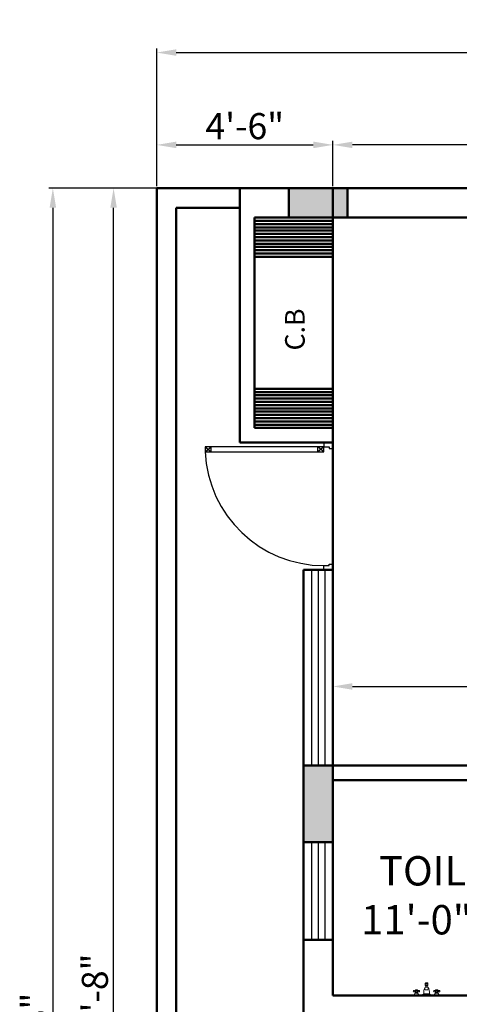
# Model space of a CAD drawing. Units: millimetres. Extents: x 1706 to 5913, y 156 to 1716.
# Tile 23 of 26: x 4554 to 4689, y 1414 to 1716. Entities that reach past the tile are written whole.
import ezdxf

# ---------------------------------------------------------------- set-up
doc = ezdxf.new("R2010")
doc.units = ezdxf.units.MM
for name, color, linetype, lineweight in [('A-ANNO-DIMS', 2, 'Continuous', 18), ('A-AREA-IDEN', 3, 'Continuous', 18), ('A-COLS', 20, 'Continuous', 50), ('A-DOOR', 4, 'Continuous', 25), ('A-FLOR-FIXT', 8, 'Continuous', 18), ('A-GLAZ', 150, 'Continuous', 25), ('A-WALL', 7, 'Continuous', 50)]:
    doc.layers.add(name, color=color, linetype=linetype, lineweight=lineweight)
doc.styles.get("Standard").update_dxf_attribs({"font": 'arial.ttf'})
doc.dimstyles.new('ISO-25', dxfattribs={"dimtxt": 8, "dimasz": 6, "dimexe": 1.25, "dimexo": 0.625, "dimtad": 1, "dimdec": 0, "dimlunit": 3, "dimtxsty": 'Standard', "dimcen": 2.5, "dimadec": 0, "dimazin": 0, "dimtfac": 1, "dimtdec": 0, "dimtmove": 0, "dimatfit": 3, "dimfxl": 1, "dimarcsym": 0})

# ---------------------------------------------------------------- blocks, each defined once
blk = doc.blocks.new('Puerta 01')
for p, q in [((-0.7745, -0.0264), (-0.7368, -0.0584)), ((-0.7745, -0.0584), (-0.7368, -0.0264)), ((-0.7368, -0.0584), (-0.7368, -0.0264)), ((-0.028, -0.0584), (-0.0657, -0.0264)), ((-0.028, -0.0264), (-0.0657, -0.0584)), ((-0.0657, -0.0584), (-0.0657, -0.0264))]:
    blk.add_line(p, q)
for points in [[(-0.028, 0), (-0.028, -0.0264), (0.004, -0.0264), (0.004, -0.036), (0.028, -0.036), (0.028, 0)], [(-0.028, -0.0264), (-0.7745, -0.0264), (-0.7745, -0.0584), (-0.028, -0.0584)], [(0.004, -0.7736), (0.004, -0.764), (0.028, -0.764), (0.028, -0.8), (-0.028, -0.8), (-0.028, -0.7736)]]:
    blk.add_lwpolyline(points, close=True)
blk.add_arc((-0.028, -0.0264), 0.7472, 182.45453, 270)
blk = doc.blocks.new('Faucet - Bathroom front')
for p, q in [((-0.5, 4.25), (0.5, 4.25)), ((0.5, 3.75), (-0.5, 3.75)), ((-5, 0), (-2.25, 0)), ((-4.5087, 0.25), (-2.7408, 0.25)), ((-4, 1.625), (-4.25, 1.625)), ((-4, 1.375), (-4.25, 1.375)), ((-3.1442, 0.75), (-4.0979, 0.75)), ((-3.25, 1.625), (-3, 1.625)), ((-3.25, 1.375), (-3, 1.375)), ((-1.5, 0), (1.5, 0)), ((-1, 0.5), (1, 0.5)), ((-0.5, 3), (0.5, 3)), ((0.5, 2), (-0.5, 2)), ((-0.25, 3), (-0.25, 3.5)), ((0.25, 3.5), (0.25, 3)), ((2.25, 0), (5, 0)), ((2.7413, 0.25), (4.5092, 0.25)), ((3.25, 1.625), (3, 1.625)), ((3.25, 1.375), (3, 1.375)), ((4.1058, 0.75), (3.1521, 0.75)), ((4, 1.625), (4.25, 1.625)), ((4, 1.375), (4.25, 1.375))]:
    blk.add_line(p, q)
for points in [[(-0.5, 3.75), (-0.5, 4.25)], [(-0.25, 4.5), (0.25, 4.5)], [(0.5, 4.25), (0.5, 3.75)], [(0.25, 3.5), (-0.25, 3.5)]]:
    blk.add_lwpolyline(points)
for points in [[(-4, 1), (-4, 2), (-3.25, 2), (-3.25, 1)], [(3.25, 1), (3.25, 2), (4, 2), (4, 1)]]:
    blk.add_lwpolyline(points, close=True)
for centre in [(-4.5, 1.5), (-3.625, 1.5), (-2.75, 1.5), (2.75, 1.5), (3.625, 1.5), (4.5, 1.5)]:
    blk.add_circle(centre, 0.2795)
for centre, radius, start, end in [((-0.2575, 4.2575), 0.2426, 88.22243, 181.7776), ((-0.2575, 3.7425), 0.2426, 178.2224, 271.7776), ((0.2575, 4.2575), 0.2426, 358.2224, 91.77757), ((0.2575, 3.7425), 0.2426, 268.2224, 1.777565), ((-5.375, 1.375), 1.4252, 285.2551, 344.7449), ((-1.875, 1.375), 1.4252, 195.2551, 254.7449), ((-0.7962, -0.2038), 0.7327, 106.1502, 163.8498), ((3, 1), 4.0311, 150.2551, 187.125), ((0.6413, 2.5), 1.246, 156.3417, 203.6583), ((-3, 1), 4.0311, 352.875, 29.74488), ((-0.6413, 2.5), 1.246, 336.3417, 23.65835), ((0.7962, -0.2038), 0.7327, 16.1502, 73.84979), ((1.875, 1.375), 1.4252, 285.2551, 344.7449), ((5.375, 1.375), 1.4252, 195.2551, 254.7449)]:
    blk.add_arc(centre, radius, start, end)
blk = doc.blocks.new('*D78')
at = {"layer": 'A-ANNO-DIMS', "color": 0, "lineweight": -2, "transparency": 16777216}
for p, q in [((4650.38, 1527.55), (4650.38, 1510.16)), ((4930.88, 1527.55), (4930.88, 1510.16)), ((4656.38, 1511.41), (4924.88, 1511.41))]:
    blk.add_line(p, q, dxfattribs=at)
at = {"layer": 'A-ANNO-DIMS', "color": 0, "transparency": 16777216}
for points in [[(4656.38, 1512.41), (4656.38, 1510.41), (4650.38, 1511.41)], [(4924.88, 1512.41), (4924.88, 1510.41), (4930.88, 1511.41)]]:
    blk.add_solid(points, dxfattribs=at)
at = {"layer": 'Defpoints', "color": 0, "transparency": 16777216}
for p in [(4650.38, 1528.17), (4930.88, 1528.17), (4930.88, 1511.41)]:
    blk.add_point(p, dxfattribs=at)
at = {"layer": 'A-ANNO-DIMS', "color": 0, "transparency": 16777216, "insert": (4790.63, 1516.12), "char_height": 8, "attachment_point": 5}
blk.add_mtext('23\'-5"', dxfattribs=at)
blk = doc.blocks.new('*D116')
at = {"layer": 'A-ANNO-DIMS', "color": 0, "lineweight": -2, "transparency": 16777216}
for p, q in [((4596.38, 1664.81), (4596.38, 1678.72)), ((4650.38, 1664.81), (4650.38, 1678.72)), ((4602.38, 1677.47), (4644.38, 1677.47))]:
    blk.add_line(p, q, dxfattribs=at)
at = {"layer": 'A-ANNO-DIMS', "color": 0, "transparency": 16777216}
for points in [[(4602.38, 1678.47), (4602.38, 1676.47), (4596.38, 1677.47)], [(4644.38, 1678.47), (4644.38, 1676.47), (4650.38, 1677.47)]]:
    blk.add_solid(points, dxfattribs=at)
at = {"layer": 'Defpoints', "color": 0, "transparency": 16777216}
for p in [(4650.38, 1677.47), (4596.38, 1664.18), (4650.38, 1664.18)]:
    blk.add_point(p, dxfattribs=at)
at = {"layer": 'A-ANNO-DIMS', "color": 0, "transparency": 16777216, "insert": (4623.38, 1682.18), "char_height": 8, "attachment_point": 5}
blk.add_mtext('4\'-6"', dxfattribs=at)
blk = doc.blocks.new('*D113')
at = {"layer": 'A-ANNO-DIMS', "color": 0, "lineweight": -2, "transparency": 16777216}
for p, q in [((4650.38, 1664.81), (4650.38, 1678.72)), ((5352.49, 1664.81), (5352.49, 1678.72)), ((5346.49, 1677.47), (4656.38, 1677.47))]:
    blk.add_line(p, q, dxfattribs=at)
at = {"layer": 'A-ANNO-DIMS', "color": 0, "transparency": 16777216}
for points in [[(4656.38, 1678.47), (4656.38, 1676.47), (4650.38, 1677.47)], [(5346.49, 1678.47), (5346.49, 1676.47), (5352.49, 1677.47)]]:
    blk.add_solid(points, dxfattribs=at)
at = {"layer": 'Defpoints', "color": 0, "transparency": 16777216}
for p in [(4650.38, 1677.47), (4650.38, 1664.18), (5352.49, 1664.18)]:
    blk.add_point(p, dxfattribs=at)
at = {"layer": 'A-ANNO-DIMS', "color": 0, "transparency": 16777216, "insert": (5001.44, 1682.18), "char_height": 8, "attachment_point": 5}
blk.add_mtext('58\'-6"', dxfattribs=at)
blk = doc.blocks.new('*D115')
at = {"layer": 'A-ANNO-DIMS', "color": 0, "lineweight": -2, "transparency": 16777216}
for p, q in [((4596.38, 1664.81), (4596.38, 1707.03)), ((5491.67, 1664.81), (5491.67, 1707.03)), ((4602.38, 1705.78), (5485.67, 1705.78))]:
    blk.add_line(p, q, dxfattribs=at)
at = {"layer": 'A-ANNO-DIMS', "color": 0, "transparency": 16777216}
for points in [[(4602.38, 1706.78), (4602.38, 1704.78), (4596.38, 1705.78)], [(5485.67, 1706.78), (5485.67, 1704.78), (5491.67, 1705.78)]]:
    blk.add_solid(points, dxfattribs=at)
at = {"layer": 'Defpoints', "color": 0, "transparency": 16777216}
for p in [(5491.67, 1705.78), (4596.38, 1664.18), (5491.67, 1664.18)]:
    blk.add_point(p, dxfattribs=at)
at = {"layer": 'A-ANNO-DIMS', "color": 0, "transparency": 16777216, "insert": (5044.03, 1710.41), "char_height": 8, "attachment_point": 5}
blk.add_mtext('74\'-7"', dxfattribs=at)
blk = doc.blocks.new('*D117')
at = {"layer": 'A-ANNO-DIMS', "color": 0, "lineweight": -2, "transparency": 16777216}
for p, q in [((4595.76, 1664.18), (4563.3, 1664.18)), ((4564.55, 1658.18), (4564.55, 1146.68)), ((4595.76, 1140.68), (4563.3, 1140.68))]:
    blk.add_line(p, q, dxfattribs=at)
at = {"layer": 'A-ANNO-DIMS', "color": 0, "transparency": 16777216}
for points in [[(4563.55, 1658.18), (4565.55, 1658.18), (4564.55, 1664.18)], [(4563.55, 1146.68), (4565.55, 1146.68), (4564.55, 1140.68)]]:
    blk.add_solid(points, dxfattribs=at)
at = {"layer": 'Defpoints', "color": 0, "transparency": 16777216}
for p in [(4596.38, 1664.18), (4564.55, 1140.68), (4596.38, 1140.68)]:
    blk.add_point(p, dxfattribs=at)
at = {"layer": 'A-ANNO-DIMS', "color": 0, "transparency": 16777216, "insert": (4559.84, 1402.43), "char_height": 8, "attachment_point": 5, "rotation": 90}
blk.add_mtext('43\'-8"', dxfattribs=at)
blk = doc.blocks.new('*D118')
at = {"layer": 'A-ANNO-DIMS', "color": 0, "lineweight": -2, "transparency": 16777216}
for p, q in [((4621.26, 1664.18), (4581.92, 1664.18)), ((4583.17, 1170.68), (4583.17, 1658.18)), ((4621.26, 1164.68), (4581.92, 1164.68))]:
    blk.add_line(p, q, dxfattribs=at)
at = {"layer": 'A-ANNO-DIMS', "color": 0, "transparency": 16777216}
for points in [[(4582.17, 1658.18), (4584.17, 1658.18), (4583.17, 1664.18)], [(4582.17, 1170.68), (4584.17, 1170.68), (4583.17, 1164.68)]]:
    blk.add_solid(points, dxfattribs=at)
at = {"layer": 'Defpoints', "color": 0, "transparency": 16777216}
for p in [(4583.17, 1664.18), (4621.88, 1664.18), (4621.88, 1164.68)]:
    blk.add_point(p, dxfattribs=at)
at = {"layer": 'A-ANNO-DIMS', "color": 0, "transparency": 16777216, "insert": (4578.46, 1414.43), "char_height": 8, "attachment_point": 5, "rotation": 90}
blk.add_mtext('41\'-8"', dxfattribs=at)

msp = doc.modelspace()

# ---------------------------------------------------------------- hatches: boundary and pattern name
at = {"layer": 'A-COLS'}
h = msp.add_hatch(color=256, dxfattribs=at)
h.dxf.hatch_style = 1
h.paths.add_polyline_path([(4654.88, 1664.18), (4636.88, 1664.18), (4636.88, 1655.18), (4654.88, 1655.18)])
h = msp.add_hatch(color=256, dxfattribs=at)
h.dxf.hatch_style = 1
h.paths.add_polyline_path([(4650.38, 1487.18), (4641.38, 1487.18), (4641.38, 1463.68), (4650.38, 1463.68)])

# ---------------------------------------------------------------- linework, layer by layer
msp.add_lwpolyline([(4655.1, 1664.18), (4636.88, 1664.18), (4636.88, 1655.18), (4654.88, 1655.18), (4654.88, 1664.18)], dxfattribs=at)
msp.add_lwpolyline([(4650.38, 1487.18), (4641.38, 1487.18), (4641.38, 1463.68), (4650.38, 1463.68)], close=True, dxfattribs=at)
at = {"layer": 'A-GLAZ'}
for p, q in [((4643.88, 1547.18), (4643.88, 1487.18)), ((4645.88, 1547.18), (4645.88, 1487.18)), ((4647.88, 1547.18), (4647.88, 1487.18)), ((4643.88, 1463.68), (4643.88, 1433.68)), ((4645.88, 1463.68), (4645.88, 1433.68)), ((4647.88, 1463.68), (4647.88, 1433.68))]:
    msp.add_line(p, q, dxfattribs=at)
for points in [[(4650.38, 1487.18), (4641.38, 1487.18), (4641.38, 1547.18), (4650.38, 1547.18)], [(4650.38, 1433.68), (4641.38, 1433.68), (4641.38, 1463.68), (4650.38, 1463.68)]]:
    msp.add_lwpolyline(points, close=True, dxfattribs=at)
at = {"layer": 'A-WALL'}
for p, q in [((4596.38, 1664.18), (4596.38, 1140.68)), ((4596.38, 1664.18), (4621.88, 1664.18)), ((4621.88, 1664.18), (4621.88, 1586.18)), ((4621.88, 1664.18), (5436.38, 1664.18)), ((4650.38, 1664.18), (4650.38, 1487.18)), ((4654.88, 1664.18), (4654.88, 1655.18)), ((4654.88, 1655.18), (4654.88, 1664.18)), ((4602.38, 1658.18), (4602.38, 1170.68)), ((4602.38, 1658.18), (4621.88, 1658.18)), ((4626.38, 1655.18), (4626.38, 1590.68)), ((4626.38, 1655.18), (5023.88, 1655.18)), ((4626.38, 1654.18), (4650.38, 1654.18)), ((4626.38, 1653.18), (4650.38, 1653.18)), ((4626.38, 1652.18), (4650.38, 1652.18)), ((4626.38, 1651.18), (4650.38, 1651.18)), ((4626.38, 1650.18), (4650.38, 1650.18)), ((4626.38, 1649.18), (4650.38, 1649.18)), ((4626.38, 1648.18), (4650.38, 1648.18)), ((4626.38, 1647.18), (4650.38, 1647.18)), ((4626.38, 1646.18), (4650.38, 1646.18)), ((4626.38, 1645.18), (4650.38, 1645.18)), ((4626.38, 1644.18), (4650.38, 1644.18)), ((4626.38, 1643.18), (4650.38, 1643.18)), ((4626.38, 1602.68), (4650.38, 1602.68)), ((4626.38, 1601.68), (4650.38, 1601.68)), ((4626.38, 1600.68), (4650.38, 1600.68)), ((4626.38, 1599.68), (4650.38, 1599.68)), ((4626.38, 1598.68), (4650.38, 1598.68)), ((4626.38, 1597.68), (4650.38, 1597.68)), ((4626.38, 1596.68), (4650.38, 1596.68)), ((4626.38, 1595.68), (4650.38, 1595.68)), ((4626.38, 1594.68), (4650.38, 1594.68)), ((4626.38, 1593.68), (4650.38, 1593.68)), ((4626.38, 1592.68), (4650.38, 1592.68)), ((4626.38, 1591.68), (4650.38, 1591.68)), ((4626.38, 1590.68), (4650.38, 1590.68)), ((4621.88, 1586.18), (4650.38, 1586.18)), ((4641.38, 1547.18), (4641.38, 1281.68)), ((4641.38, 1547.18), (4650.38, 1547.18)), ((4650.38, 1487.18), (4849.88, 1487.18)), ((4650.38, 1482.68), (4650.38, 1416.68)), ((4650.38, 1482.68), (4849.88, 1482.68)), ((4641.38, 1463.68), (4650.38, 1463.68)), ((4641.38, 1433.68), (4650.38, 1433.68)), ((4650.38, 1416.68), (4782.38, 1416.68))]:
    msp.add_line(p, q, dxfattribs=at)

# ---------------------------------------------------------------- block references
at = {"layer": 'A-DOOR', "xscale": 48.75000000000287, "yscale": 48.75000000000287, "zscale": 48.75000000000287}
msp.add_blockref('Puerta 01', (4649.02, 1586.18), dxfattribs=at)
at = {"layer": 'A-FLOR-FIXT', "xscale": 0.8570205523683982, "yscale": 0.8570205523683982, "zscale": 0.8570205523683982}
msp.add_blockref('Faucet - Bathroom front', (4679.1, 1416.68), dxfattribs=at)

# ---------------------------------------------------------------- texts
at = {"layer": 'A-AREA-IDEN', "insert": (4635.74, 1605.26), "char_height": 6, "attachment_point": 1, "rotation": 90}
msp.add_mtext_dynamic_manual_height_columns('     C.B', width=33.9892, gutter_width=12.5, heights=[0], dxfattribs=at)
at = {"layer": 'A-AREA-IDEN', "insert": (4653.53, 1459.38), "char_height": 9, "attachment_point": 1}
msp.add_mtext_dynamic_manual_height_columns('    TOILET\\P  11\'-0"X5\'-6"', width=90.4844, gutter_width=12.5, heights=[0], dxfattribs=at)

# ---------------------------------------------------------------- dimensions: what is measured, and where the dimension line sits
at = {"layer": 'A-ANNO-DIMS'}
for base, p1, p2, picture, middle in [((5491.67, 1705.78), (4596.38, 1664.18), (5491.67, 1664.18), '*D115', (5044.03, 1710.41)), ((4650.38, 1677.47), (4596.38, 1664.18), (4650.38, 1664.18), '*D116', (4623.38, 1682.18)), ((4650.38, 1677.47), (5352.49, 1664.18), (4650.38, 1664.18), '*D113', (5001.44, 1682.18)), ((4930.88109307, 1511.4081474), (4650.38109307, 1528.17377043), (4930.88109307, 1528.17377043), '*D78', (4790.63109307, 1516.12045982))]:
    dim = msp.add_linear_dim(base=base, p1=p1, p2=p2, dimstyle='ISO-25', override={"dimclrd": 0, "dimclre": 0, "dimclrt": 0}, dxfattribs=at)
    dim.commit()
    dim.dimension.update_dxf_attribs({"geometry": picture, "text_midpoint": middle})
for base, p1, p2, picture, middle in [((4564.55212222, 1140.68004162), (4596.38109307, 1664.18004162), (4596.38109307, 1140.68004162), '*D117', (4559.83980981, 1402.43004162)), ((4583.16597931, 1664.18004162), (4621.88109307, 1164.68004162), (4621.88109307, 1664.18004162), '*D118', (4578.45639541, 1414.43004162))]:
    dim = msp.add_linear_dim(base=base, p1=p1, p2=p2, angle=90, dimstyle='ISO-25', override={"dimclrd": 0, "dimclre": 0, "dimclrt": 0}, dxfattribs=at)
    dim.commit()
    dim.dimension.update_dxf_attribs({"geometry": picture, "text_midpoint": middle})

doc.saveas('drawing.dxf')
